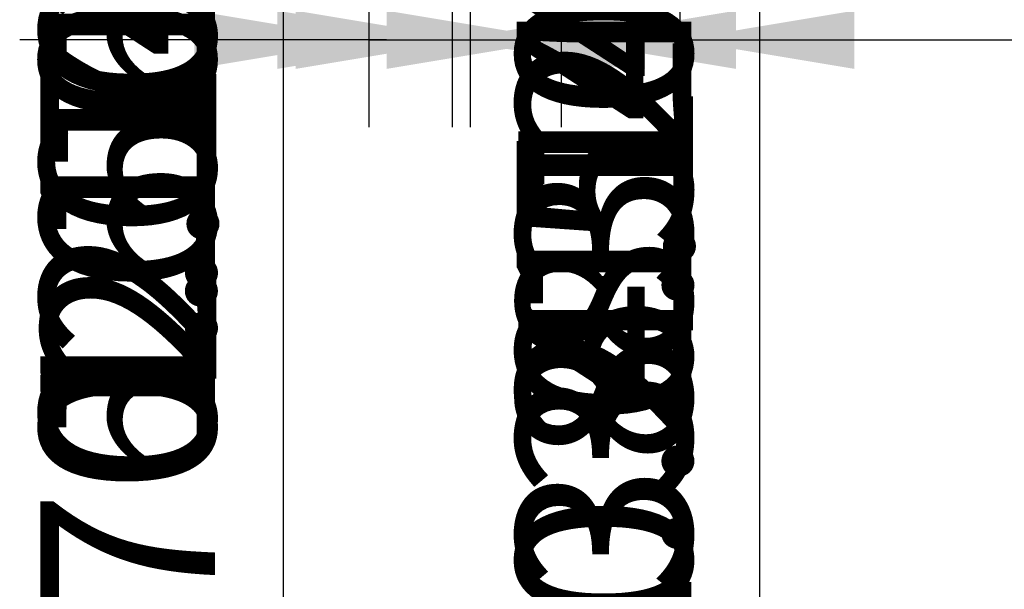
# Model space of a CAD drawing. Units: metres. Extents: x 782 to 1487, y 1262 to 7446.
# Tile 4 of 25: x 807.13 to 821.23, y 1279.51 to 1287.66. Entities that reach past the tile are written whole.
import ezdxf

# ---------------------------------------------------------------- set-up
doc = ezdxf.new("R2010")
doc.units = ezdxf.units.M
doc.layers.add('A-ANNO-DIMS', color=2, linetype='Continuous', lineweight=18)
doc.styles.get("Standard").update_dxf_attribs({"font": 'arial.ttf'})
doc.dimstyles.new('ISO-25', dxfattribs={"dimtxt": 2.5, "dimasz": 2.5, "dimexe": 1.25, "dimexo": 0.625, "dimtad": 1, "dimtxsty": 'Standard', "dimcen": 2.5, "dimadec": 0, "dimazin": 0, "dimtfac": 1, "dimtmove": 0, "dimatfit": 3, "dimfxl": 1, "dimarcsym": 0})

# ---------------------------------------------------------------- blocks, each defined once
blk = doc.blocks.new('*D10')
at = {"layer": 'A-ANNO-DIMS', "color": 0, "lineweight": -2, "transparency": 16777216}
for p, q in [((825.73, 1277.527), (825.73, 1276.166)), ((826.753, 1277.552), (826.753, 1276.166)), ((823.23, 1277.416), (820.73, 1277.416)), ((825.73, 1277.416), (826.753, 1277.416)), ((829.253, 1277.416), (839.235, 1277.416))]:
    blk.add_line(p, q, dxfattribs=at)
at = {"layer": 'A-ANNO-DIMS', "color": 0, "transparency": 16777216}
for points in [[(823.23, 1277.833), (823.23, 1276.999), (825.73, 1277.416)], [(829.253, 1277.833), (829.253, 1276.999), (826.753, 1277.416)]]:
    blk.add_solid(points, dxfattribs=at)
at = {"layer": 'Defpoints', "color": 0, "transparency": 16777216}
for p in [(825.73, 1278.152), (826.753, 1278.177), (826.753, 1277.416)]:
    blk.add_point(p, dxfattribs=at)
at = {"layer": 'A-ANNO-DIMS', "color": 0, "transparency": 16777216, "insert": (835.494, 1279.543), "char_height": 2.5, "attachment_point": 5}
blk.add_mtext('1,02', dxfattribs=at)
blk = doc.blocks.new('*D56')
at = {"layer": 'A-ANNO-DIMS', "color": 0, "lineweight": -2, "transparency": 16777216}
for p, q in [((810.9, 1304.677), (810.9, 1307.177)), ((811.735, 1302.177), (809.65, 1302.177)), ((810.9, 1302.177), (810.9, 1299.809)), ((811.505, 1299.809), (809.65, 1299.809)), ((810.9, 1297.309), (810.9, 1287.022))]:
    blk.add_line(p, q, dxfattribs=at)
at = {"layer": 'A-ANNO-DIMS', "color": 0, "transparency": 16777216}
for points in [[(810.483, 1304.677), (811.317, 1304.677), (810.9, 1302.177)], [(810.483, 1297.309), (811.317, 1297.309), (810.9, 1299.809)]]:
    blk.add_solid(points, dxfattribs=at)
at = {"layer": 'Defpoints', "color": 0, "transparency": 16777216}
for p in [(812.36, 1302.177), (810.9, 1299.809), (812.13, 1299.809)]:
    blk.add_point(p, dxfattribs=at)
at = {"layer": 'A-ANNO-DIMS', "color": 0, "transparency": 16777216, "insert": (808.998, 1290.916), "char_height": 2.5, "attachment_point": 5, "rotation": 90}
blk.add_mtext('2.37', dxfattribs=at)
blk = doc.blocks.new('*D57')
at = {"layer": 'A-ANNO-DIMS', "color": 0, "lineweight": -2, "transparency": 16777216}
for p, q in [((810.9, 1302.309), (810.9, 1304.809)), ((811.505, 1299.809), (809.65, 1299.809)), ((810.9, 1299.809), (810.9, 1298.647)), ((811.735, 1298.647), (809.65, 1298.647)), ((810.9, 1296.147), (810.9, 1286.141))]:
    blk.add_line(p, q, dxfattribs=at)
at = {"layer": 'A-ANNO-DIMS', "color": 0, "transparency": 16777216}
for points in [[(810.483, 1302.309), (811.317, 1302.309), (810.9, 1299.809)], [(810.483, 1296.147), (811.317, 1296.147), (810.9, 1298.647)]]:
    blk.add_solid(points, dxfattribs=at)
at = {"layer": 'Defpoints', "color": 0, "transparency": 16777216}
for p in [(812.13, 1299.809), (810.9, 1298.647), (812.36, 1298.647)]:
    blk.add_point(p, dxfattribs=at)
at = {"layer": 'A-ANNO-DIMS', "color": 0, "transparency": 16777216, "insert": (808.999, 1289.894), "char_height": 2.5, "attachment_point": 5, "rotation": 90}
blk.add_mtext('1.16', dxfattribs=at)
blk = doc.blocks.new('*D58')
at = {"layer": 'A-ANNO-DIMS', "color": 0, "lineweight": -2, "transparency": 16777216}
for p, q in [((810.9, 1301.147), (810.9, 1303.647)), ((811.735, 1298.647), (809.65, 1298.647)), ((810.9, 1298.647), (810.9, 1296.5)), ((811.507, 1296.5), (809.65, 1296.5)), ((810.9, 1294), (810.9, 1281.772))]:
    blk.add_line(p, q, dxfattribs=at)
at = {"layer": 'A-ANNO-DIMS', "color": 0, "transparency": 16777216}
for points in [[(810.483, 1301.147), (811.317, 1301.147), (810.9, 1298.647)], [(810.483, 1294), (811.317, 1294), (810.9, 1296.5)]]:
    blk.add_solid(points, dxfattribs=at)
at = {"layer": 'Defpoints', "color": 0, "transparency": 16777216}
for p in [(812.36, 1298.647), (810.9, 1296.5), (812.132, 1296.5)]:
    blk.add_point(p, dxfattribs=at)
at = {"layer": 'A-ANNO-DIMS', "color": 0, "transparency": 16777216, "insert": (809.02, 1286.636), "char_height": 2.5, "attachment_point": 5, "rotation": 90}
blk.add_mtext('2.147', dxfattribs=at)
blk = doc.blocks.new('*D59')
at = {"layer": 'A-ANNO-DIMS', "color": 0, "lineweight": -2, "transparency": 16777216}
for p, q in [((810.9, 1299), (810.9, 1301.5)), ((811.507, 1296.5), (809.65, 1296.5)), ((810.9, 1296.5), (810.9, 1295.397)), ((811.735, 1295.397), (809.65, 1295.397)), ((810.9, 1292.897), (810.9, 1280.947))]:
    blk.add_line(p, q, dxfattribs=at)
at = {"layer": 'A-ANNO-DIMS', "color": 0, "transparency": 16777216}
for points in [[(810.483, 1299), (811.317, 1299), (810.9, 1296.5)], [(810.483, 1292.897), (811.317, 1292.897), (810.9, 1295.397)]]:
    blk.add_solid(points, dxfattribs=at)
at = {"layer": 'Defpoints', "color": 0, "transparency": 16777216}
for p in [(812.132, 1296.5), (810.9, 1295.397), (812.36, 1295.397)]:
    blk.add_point(p, dxfattribs=at)
at = {"layer": 'A-ANNO-DIMS', "color": 0, "transparency": 16777216, "insert": (808.998, 1285.672), "char_height": 2.5, "attachment_point": 5, "rotation": 90}
blk.add_mtext('1.103', dxfattribs=at)
blk = doc.blocks.new('*D60')
at = {"layer": 'A-ANNO-DIMS', "color": 0, "lineweight": -2, "transparency": 16777216}
for p, q in [((810.9, 1297.897), (810.9, 1300.397)), ((811.735, 1295.397), (809.65, 1295.397)), ((810.9, 1295.397), (810.9, 1293.74)), ((811.505, 1293.74), (809.65, 1293.74)), ((810.9, 1291.24), (810.9, 1281.233))]:
    blk.add_line(p, q, dxfattribs=at)
at = {"layer": 'A-ANNO-DIMS', "color": 0, "transparency": 16777216}
for points in [[(810.483, 1297.897), (811.317, 1297.897), (810.9, 1295.397)], [(810.483, 1291.24), (811.317, 1291.24), (810.9, 1293.74)]]:
    blk.add_solid(points, dxfattribs=at)
at = {"layer": 'Defpoints', "color": 0, "transparency": 16777216}
for p in [(812.36, 1295.397), (810.9, 1293.74), (812.13, 1293.74)]:
    blk.add_point(p, dxfattribs=at)
at = {"layer": 'A-ANNO-DIMS', "color": 0, "transparency": 16777216, "insert": (808.999, 1284.987), "char_height": 2.5, "attachment_point": 5, "rotation": 90}
blk.add_mtext('1.66', dxfattribs=at)
blk = doc.blocks.new('*D61')
at = {"layer": 'A-ANNO-DIMS', "color": 0, "lineweight": -2, "transparency": 16777216}
for p, q in [((810.9, 1296.24), (810.9, 1298.74)), ((811.505, 1293.74), (809.65, 1293.74)), ((810.9, 1293.74), (810.9, 1293.067)), ((811.505, 1293.067), (809.65, 1293.067)), ((810.9, 1290.567), (810.9, 1280.324))]:
    blk.add_line(p, q, dxfattribs=at)
at = {"layer": 'A-ANNO-DIMS', "color": 0, "transparency": 16777216}
for points in [[(810.483, 1296.24), (811.317, 1296.24), (810.9, 1293.74)], [(810.483, 1290.567), (811.317, 1290.567), (810.9, 1293.067)]]:
    blk.add_solid(points, dxfattribs=at)
at = {"layer": 'Defpoints', "color": 0, "transparency": 16777216}
for p in [(812.13, 1293.74), (810.9, 1293.067), (812.13, 1293.067)]:
    blk.add_point(p, dxfattribs=at)
at = {"layer": 'A-ANNO-DIMS', "color": 0, "transparency": 16777216, "insert": (808.999, 1284.195), "char_height": 2.5, "attachment_point": 5, "rotation": 90}
blk.add_mtext('0.67', dxfattribs=at)
blk = doc.blocks.new('*D62')
at = {"layer": 'A-ANNO-DIMS', "color": 0, "lineweight": -2, "transparency": 16777216}
for p, q in [((810.9, 1295.567), (810.9, 1298.067)), ((811.505, 1293.067), (809.65, 1293.067)), ((810.9, 1293.067), (810.9, 1290.305)), ((811.505, 1290.305), (809.65, 1290.305)), ((810.9, 1287.805), (810.9, 1275.602))]:
    blk.add_line(p, q, dxfattribs=at)
at = {"layer": 'A-ANNO-DIMS', "color": 0, "transparency": 16777216}
for points in [[(810.483, 1295.567), (811.317, 1295.567), (810.9, 1293.067)], [(810.483, 1287.805), (811.317, 1287.805), (810.9, 1290.305)]]:
    blk.add_solid(points, dxfattribs=at)
at = {"layer": 'Defpoints', "color": 0, "transparency": 16777216}
for p in [(812.13, 1293.067), (810.9, 1290.305), (812.13, 1290.305)]:
    blk.add_point(p, dxfattribs=at)
at = {"layer": 'A-ANNO-DIMS', "color": 0, "transparency": 16777216, "insert": (808.999, 1280.454), "char_height": 2.5, "attachment_point": 5, "rotation": 90}
blk.add_mtext('2.762', dxfattribs=at)
blk = doc.blocks.new('*D64')
at = {"layer": 'A-ANNO-DIMS', "color": 0, "lineweight": -2, "transparency": 16777216}
for p, q in [((817.721, 1307.367), (817.721, 1309.867)), ((817.205, 1304.867), (818.971, 1304.867)), ((817.721, 1304.867), (817.721, 1300.338)), ((817.206, 1300.338), (818.971, 1300.338)), ((817.721, 1297.838), (817.721, 1285.546))]:
    blk.add_line(p, q, dxfattribs=at)
at = {"layer": 'A-ANNO-DIMS', "color": 0, "transparency": 16777216}
for points in [[(817.304, 1307.367), (818.138, 1307.367), (817.721, 1304.867)], [(817.304, 1297.838), (818.138, 1297.838), (817.721, 1300.338)]]:
    blk.add_solid(points, dxfattribs=at)
at = {"layer": 'Defpoints', "color": 0, "transparency": 16777216}
for p in [(816.58, 1304.867), (816.581, 1300.338), (817.721, 1300.338)]:
    blk.add_point(p, dxfattribs=at)
at = {"layer": 'A-ANNO-DIMS', "color": 0, "transparency": 16777216, "insert": (815.82, 1290.442), "char_height": 2.5, "attachment_point": 5, "rotation": 90}
blk.add_mtext('4.529', dxfattribs=at)
blk = doc.blocks.new('*D65')
at = {"layer": 'A-ANNO-DIMS', "color": 0, "lineweight": -2, "transparency": 16777216}
for p, q in [((817.721, 1302.838), (817.721, 1305.338)), ((817.206, 1300.338), (818.971, 1300.338)), ((817.721, 1300.338), (817.721, 1296.196)), ((817.205, 1296.196), (818.971, 1296.196)), ((817.721, 1293.696), (817.721, 1281.435))]:
    blk.add_line(p, q, dxfattribs=at)
at = {"layer": 'A-ANNO-DIMS', "color": 0, "transparency": 16777216}
for points in [[(817.304, 1302.838), (818.138, 1302.838), (817.721, 1300.338)], [(817.304, 1293.696), (818.138, 1293.696), (817.721, 1296.196)]]:
    blk.add_solid(points, dxfattribs=at)
at = {"layer": 'Defpoints', "color": 0, "transparency": 16777216}
for p in [(816.581, 1300.338), (816.58, 1296.196), (817.721, 1296.196)]:
    blk.add_point(p, dxfattribs=at)
at = {"layer": 'A-ANNO-DIMS', "color": 0, "transparency": 16777216, "insert": (815.841, 1286.315), "char_height": 2.5, "attachment_point": 5, "rotation": 90}
blk.add_mtext('4.142', dxfattribs=at)
blk = doc.blocks.new('*D66')
at = {"layer": 'A-ANNO-DIMS', "color": 0, "lineweight": -2, "transparency": 16777216}
for p, q in [((817.721, 1298.696), (817.721, 1301.196)), ((817.205, 1296.196), (818.971, 1296.196)), ((817.721, 1296.196), (817.721, 1293.699)), ((817.205, 1293.699), (818.971, 1293.699)), ((817.721, 1291.199), (817.721, 1280.921))]:
    blk.add_line(p, q, dxfattribs=at)
at = {"layer": 'A-ANNO-DIMS', "color": 0, "transparency": 16777216}
for points in [[(817.304, 1298.696), (818.138, 1298.696), (817.721, 1296.196)], [(817.304, 1291.199), (818.138, 1291.199), (817.721, 1293.699)]]:
    blk.add_solid(points, dxfattribs=at)
at = {"layer": 'Defpoints', "color": 0, "transparency": 16777216}
for p in [(816.58, 1296.196), (816.58, 1293.699), (817.721, 1293.699)]:
    blk.add_point(p, dxfattribs=at)
at = {"layer": 'A-ANNO-DIMS', "color": 0, "transparency": 16777216, "insert": (815.82, 1284.81), "char_height": 2.5, "attachment_point": 5, "rotation": 90}
blk.add_mtext('2.50', dxfattribs=at)
blk = doc.blocks.new('*D67')
at = {"layer": 'A-ANNO-DIMS', "color": 0, "lineweight": -2, "transparency": 16777216}
for p, q in [((817.721, 1296.199), (817.721, 1298.699)), ((817.205, 1293.699), (818.971, 1293.699)), ((817.721, 1293.699), (817.721, 1293.067)), ((817.205, 1293.067), (818.971, 1293.067)), ((817.721, 1290.567), (817.721, 1278.407))]:
    blk.add_line(p, q, dxfattribs=at)
at = {"layer": 'A-ANNO-DIMS', "color": 0, "transparency": 16777216}
for points in [[(817.304, 1296.199), (818.138, 1296.199), (817.721, 1293.699)], [(817.304, 1290.567), (818.138, 1290.567), (817.721, 1293.067)]]:
    blk.add_solid(points, dxfattribs=at)
at = {"layer": 'Defpoints', "color": 0, "transparency": 16777216}
for p in [(816.58, 1293.699), (816.58, 1293.067), (817.721, 1293.067)]:
    blk.add_point(p, dxfattribs=at)
at = {"layer": 'A-ANNO-DIMS', "color": 0, "transparency": 16777216, "insert": (815.819, 1283.237), "char_height": 2.5, "attachment_point": 5, "rotation": 90}
blk.add_mtext('0.632', dxfattribs=at)
blk = doc.blocks.new('*D68')
at = {"layer": 'A-ANNO-DIMS', "color": 0, "lineweight": -2, "transparency": 16777216}
for p, q in [((817.721, 1295.567), (817.721, 1298.067)), ((815.508, 1293.067), (818.971, 1293.067)), ((817.721, 1293.067), (817.721, 1291.686)), ((815.508, 1291.686), (818.971, 1291.686)), ((817.721, 1289.186), (817.721, 1277.718))]:
    blk.add_line(p, q, dxfattribs=at)
at = {"layer": 'A-ANNO-DIMS', "color": 0, "transparency": 16777216}
for points in [[(817.304, 1295.567), (818.138, 1295.567), (817.721, 1293.067)], [(817.304, 1289.186), (818.138, 1289.186), (817.721, 1291.686)]]:
    blk.add_solid(points, dxfattribs=at)
at = {"layer": 'Defpoints', "color": 0, "transparency": 16777216}
for p in [(814.883, 1293.067), (814.883, 1291.686), (817.721, 1291.686)]:
    blk.add_point(p, dxfattribs=at)
at = {"layer": 'A-ANNO-DIMS', "color": 0, "transparency": 16777216, "insert": (815.819, 1282.202), "char_height": 2.5, "attachment_point": 5, "rotation": 90}
blk.add_mtext('1.381', dxfattribs=at)
blk = doc.blocks.new('*D69')
at = {"layer": 'A-ANNO-DIMS', "color": 0, "lineweight": -2, "transparency": 16777216}
for p, q in [((817.721, 1294.186), (817.721, 1296.686)), ((815.508, 1291.686), (818.971, 1291.686)), ((817.721, 1291.686), (817.721, 1290.305)), ((815.508, 1290.305), (818.971, 1290.305)), ((817.721, 1287.805), (817.721, 1276.337))]:
    blk.add_line(p, q, dxfattribs=at)
at = {"layer": 'A-ANNO-DIMS', "color": 0, "transparency": 16777216}
for points in [[(817.304, 1294.186), (818.138, 1294.186), (817.721, 1291.686)], [(817.304, 1287.805), (818.138, 1287.805), (817.721, 1290.305)]]:
    blk.add_solid(points, dxfattribs=at)
at = {"layer": 'Defpoints', "color": 0, "transparency": 16777216}
for p in [(814.883, 1291.686), (814.883, 1290.305), (817.721, 1290.305)]:
    blk.add_point(p, dxfattribs=at)
at = {"layer": 'A-ANNO-DIMS', "color": 0, "transparency": 16777216, "insert": (815.819, 1280.821), "char_height": 2.5, "attachment_point": 5, "rotation": 90}
blk.add_mtext('1.381', dxfattribs=at)
blk = doc.blocks.new('*D73')
at = {"layer": 'A-ANNO-DIMS', "color": 0, "lineweight": -2, "transparency": 16777216}
for p, q in [((812.13, 1289.68), (812.13, 1286.127)), ((813.319, 1289.68), (813.319, 1286.127)), ((809.63, 1287.377), (807.13, 1287.377)), ((812.13, 1287.377), (813.319, 1287.377)), ((815.819, 1287.377), (825.832, 1287.377))]:
    blk.add_line(p, q, dxfattribs=at)
at = {"layer": 'A-ANNO-DIMS', "color": 0, "transparency": 16777216}
for points in [[(809.63, 1287.794), (809.63, 1286.96), (812.13, 1287.377)], [(815.819, 1287.794), (815.819, 1286.96), (813.319, 1287.377)]]:
    blk.add_solid(points, dxfattribs=at)
at = {"layer": 'Defpoints', "color": 0, "transparency": 16777216}
for p in [(812.13, 1290.305), (813.319, 1290.305), (813.319, 1287.377)]:
    blk.add_point(p, dxfattribs=at)
at = {"layer": 'A-ANNO-DIMS', "color": 0, "transparency": 16777216, "insert": (822.076, 1289.278), "char_height": 2.5, "attachment_point": 5}
blk.add_mtext('1.19', dxfattribs=at)
blk = doc.blocks.new('*D74')
at = {"layer": 'A-ANNO-DIMS', "color": 0, "lineweight": -2, "transparency": 16777216}
for p, q in [((813.319, 1289.68), (813.319, 1286.127)), ((813.58, 1289.68), (813.58, 1286.127)), ((810.819, 1287.377), (808.319, 1287.377)), ((813.319, 1287.377), (813.58, 1287.377)), ((816.08, 1287.377), (826.322, 1287.377))]:
    blk.add_line(p, q, dxfattribs=at)
at = {"layer": 'A-ANNO-DIMS', "color": 0, "transparency": 16777216}
for points in [[(810.819, 1287.794), (810.819, 1286.96), (813.319, 1287.377)], [(816.08, 1287.794), (816.08, 1286.96), (813.58, 1287.377)]]:
    blk.add_solid(points, dxfattribs=at)
at = {"layer": 'Defpoints', "color": 0, "transparency": 16777216}
for p in [(813.319, 1290.305), (813.58, 1290.305), (813.58, 1287.377)]:
    blk.add_point(p, dxfattribs=at)
at = {"layer": 'A-ANNO-DIMS', "color": 0, "transparency": 16777216, "insert": (822.451, 1289.278), "char_height": 2.5, "attachment_point": 5}
blk.add_mtext('0.26', dxfattribs=at)
blk = doc.blocks.new('*D75')
at = {"layer": 'A-ANNO-DIMS', "color": 0, "lineweight": -2, "transparency": 16777216}
for p, q in [((813.58, 1289.68), (813.58, 1286.127)), ((814.883, 1289.68), (814.883, 1286.127)), ((811.08, 1287.377), (808.58, 1287.377)), ((813.58, 1287.377), (814.883, 1287.377)), ((817.383, 1287.377), (827.383, 1287.377))]:
    blk.add_line(p, q, dxfattribs=at)
at = {"layer": 'A-ANNO-DIMS', "color": 0, "transparency": 16777216}
for points in [[(811.08, 1287.794), (811.08, 1286.96), (813.58, 1287.377)], [(817.383, 1287.794), (817.383, 1286.96), (814.883, 1287.377)]]:
    blk.add_solid(points, dxfattribs=at)
at = {"layer": 'Defpoints', "color": 0, "transparency": 16777216}
for p in [(813.58, 1290.305), (814.883, 1290.305), (814.883, 1287.377)]:
    blk.add_point(p, dxfattribs=at)
at = {"layer": 'A-ANNO-DIMS', "color": 0, "transparency": 16777216, "insert": (823.633, 1289.279), "char_height": 2.5, "attachment_point": 5}
blk.add_mtext('1.30', dxfattribs=at)
blk = doc.blocks.new('*D76')
at = {"layer": 'A-ANNO-DIMS', "color": 0, "lineweight": -2, "transparency": 16777216}
for p, q in [((814.883, 1289.68), (814.883, 1286.127)), ((816.58, 1289.68), (816.58, 1286.127)), ((812.383, 1287.377), (809.883, 1287.377)), ((814.883, 1287.377), (816.58, 1287.377)), ((819.08, 1287.377), (831.031, 1287.377))]:
    blk.add_line(p, q, dxfattribs=at)
at = {"layer": 'A-ANNO-DIMS', "color": 0, "transparency": 16777216}
for points in [[(812.383, 1287.794), (812.383, 1286.96), (814.883, 1287.377)], [(819.08, 1287.794), (819.08, 1286.96), (816.58, 1287.377)]]:
    blk.add_solid(points, dxfattribs=at)
at = {"layer": 'Defpoints', "color": 0, "transparency": 16777216}
for p in [(814.883, 1290.305), (816.58, 1290.305), (816.58, 1287.377)]:
    blk.add_point(p, dxfattribs=at)
at = {"layer": 'A-ANNO-DIMS', "color": 0, "transparency": 16777216, "insert": (826.305, 1289.278), "char_height": 2.5, "attachment_point": 5}
blk.add_mtext('1.697', dxfattribs=at)

msp = doc.modelspace()

# ---------------------------------------------------------------- dimensions: what is measured, and where the dimension line sits
at = {"layer": 'A-ANNO-DIMS'}
for base, p1, p2, override, picture, middle in [((817.7211, 1300.3378), (816.5802, 1304.8669), (816.5811, 1300.3378), {"dimdec": 3, "dimlfac": 1, "dimrnd": 0, "dimzin": 0, "dimdsep": 46, "dimlunit": 2}, '*D64', (815.8196, 1290.4419)), ((810.9, 1299.8088), (812.36, 1302.1774), (812.1301, 1299.8088), {"dimdec": 2, "dimlfac": 1, "dimrnd": 0, "dimzin": 0, "dimdsep": 46, "dimlunit": 2}, '*D56', (808.9978, 1290.9156)), ((817.7211, 1296.196), (816.5811, 1300.3378), (816.58, 1296.196), {"dimdec": 3, "dimlfac": 1, "dimrnd": 0, "dimzin": 0, "dimdsep": 46, "dimlunit": 2}, '*D65', (815.8409, 1286.3153)), ((810.9, 1298.6474), (812.1301, 1299.8088), (812.36, 1298.6474), {"dimdec": 2, "dimlfac": 1, "dimrnd": 0, "dimzin": 0, "dimdsep": 46, "dimlunit": 2}, '*D57', (808.9986, 1289.894)), ((810.9, 1296.5004), (812.36, 1298.6474), (812.1317, 1296.5004), {"dimdec": 3, "dimlfac": 1, "dimrnd": 0, "dimzin": 0, "dimdsep": 46, "dimlunit": 2}, '*D58', (809.0199, 1286.636)), ((810.9, 1295.3974), (812.1317, 1296.5004), (812.36, 1295.3974), {"dimdec": 3, "dimlfac": 1, "dimrnd": 0, "dimzin": 0, "dimdsep": 46, "dimlunit": 2}, '*D59', (808.9978, 1285.672)), ((817.7211, 1293.6994), (816.58, 1296.196), (816.58, 1293.6994), {"dimdec": 2, "dimlfac": 1, "dimrnd": 0, "dimzin": 0, "dimdsep": 46, "dimlunit": 2}, '*D66', (815.8196, 1284.8104)), ((810.9, 1293.7402), (812.36, 1295.3974), (812.1297, 1293.7402), {"dimdec": 2, "dimlfac": 1, "dimrnd": 0, "dimzin": 0, "dimdsep": 46, "dimlunit": 2}, '*D60', (808.9986, 1284.9868)), ((810.9, 1293.0674), (812.1297, 1293.7402), (812.13, 1293.0674), {"dimdec": 2, "dimlfac": 1, "dimrnd": 0, "dimzin": 0, "dimdsep": 46, "dimlunit": 2}, '*D61', (808.9986, 1284.1955)), ((817.7211, 1293.0674), (816.58, 1293.6994), (816.58, 1293.0674), {"dimdec": 3, "dimlfac": 1, "dimrnd": 0, "dimzin": 0, "dimdsep": 46, "dimlunit": 2}, '*D67', (815.8188, 1283.2371)), ((810.9, 1290.3053), (812.13, 1293.0674), (812.13, 1290.3053), {"dimdec": 3, "dimlfac": 1, "dimrnd": 0, "dimzin": 0, "dimdsep": 46, "dimlunit": 2}, '*D62', (808.9986, 1280.4536)), ((817.7211, 1291.6863), (814.8832, 1293.0674), (814.8832, 1291.6863), {"dimdec": 3, "dimlfac": 1, "dimrnd": 0, "dimzin": 0, "dimdsep": 46, "dimlunit": 2}, '*D68', (815.8188, 1282.2022)), ((817.7211, 1290.3053), (814.8832, 1291.6863), (814.8832, 1290.3053), {"dimdec": 3, "dimlfac": 1, "dimrnd": 0, "dimzin": 0, "dimdsep": 46, "dimlunit": 2}, '*D69', (815.8188, 1280.8211))]:
    dim = msp.add_linear_dim(base=base, p1=p1, p2=p2, angle=90, dimstyle='ISO-25', override=override, dxfattribs=at)
    dim.commit()
    dim.dimension.update_dxf_attribs({"geometry": picture, "text_midpoint": middle})
for base, p1, p2, override, picture, middle in [((813.3188, 1287.377), (812.13, 1290.3053), (813.3188, 1290.3053), {"dimdec": 2, "dimlfac": 1, "dimrnd": 0, "dimzin": 0, "dimdsep": 46, "dimlunit": 2}, '*D73', (822.0757, 1289.2784)), ((813.5796, 1287.377), (813.3188, 1290.3053), (813.5796, 1290.3053), {"dimdec": 2, "dimlfac": 1, "dimrnd": 0, "dimzin": 0, "dimdsep": 46, "dimlunit": 2}, '*D74', (822.4506, 1289.2784)), ((814.8832, 1287.377), (813.5796, 1290.3053), (814.8832, 1290.3053), {"dimdec": 2, "dimlfac": 1, "dimrnd": 0, "dimzin": 0, "dimdsep": 46, "dimlunit": 2}, '*D75', (823.6332, 1289.2792)), ((816.58, 1287.377), (814.8832, 1290.3053), (816.58, 1290.3053), {"dimdec": 3, "dimlfac": 1, "dimrnd": 0, "dimzin": 0, "dimdsep": 46, "dimlunit": 2}, '*D76', (826.3055, 1289.2784))]:
    dim = msp.add_linear_dim(base=base, p1=p1, p2=p2, dimstyle='ISO-25', override=override, dxfattribs=at)
    dim.commit()
    dim.dimension.update_dxf_attribs({"geometry": picture, "text_midpoint": middle})
dim = msp.add_linear_dim(base=(826.7525, 1277.4159), p1=(825.7296, 1278.1516), p2=(826.7525, 1278.177), dimstyle='ISO-25', override={"dimclrd": 0, "dimclre": 0, "dimclrt": 0}, dxfattribs=at)
dim.commit()
dim.dimension.update_dxf_attribs({"geometry": '*D10', "text_midpoint": (835.494, 1277.4159), "dimtype": 160})

doc.saveas('drawing.dxf')
